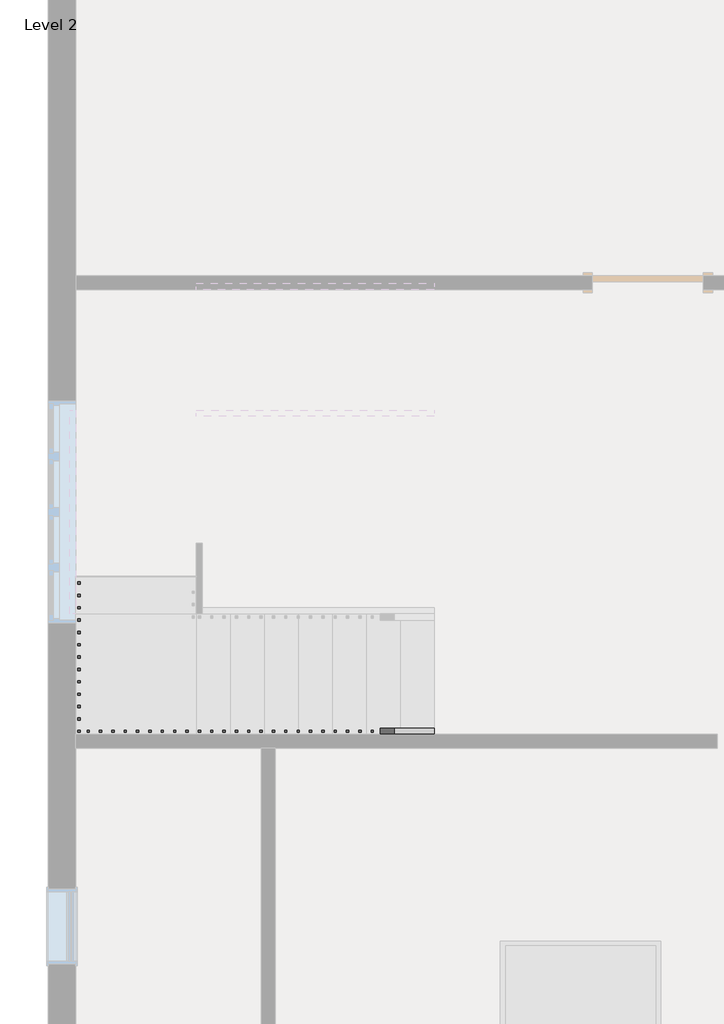
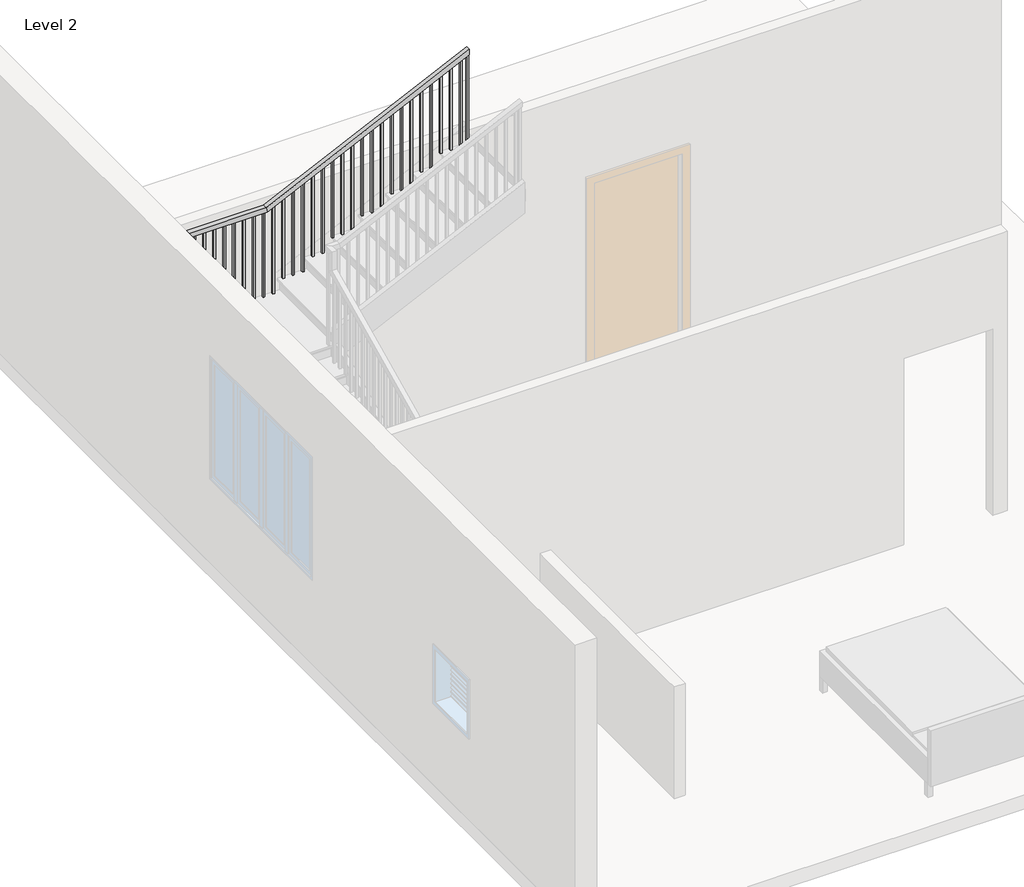
# One storey, part 2 of 3: 1 railing.
"""IFC4 building model written with IfcOpenShell, lengths in millimetres."""

from ifc_helpers import new_model, si_unit, frame, origin, place, context, project, spatial, polyline, outline, extrude, faceted_brep, element, save

model = new_model("IFC4")

# Units and contexts
model_context = context("Model", 3, world=origin())
ifc_project = project(units=[si_unit("LENGTHUNIT", "METRE", prefix="MILLI")], contexts=[model_context])

# Site, building, storey
site = spatial("IfcSite", under=ifc_project)
building = spatial("IfcBuilding", under=site)
storey = spatial("IfcBuildingStorey", under=building, Name="Level 2", Elevation=3048.0)

# Railing
placement = place(None, origin())
element("IfcRailing", 1, ObjectType="Handrail - Rectangular", at=placement, inside=storey, context=model_context, shape_type="SolidModel", body=[
    faceted_brep([(-19769.8789184, -1118.4399287, 4094.9217391), (-19769.8789184, -1118.4399287, 4038.6971684), (-19769.8789184, -1067.6399287, 4038.6971684), (-19769.8789184, -1067.6399287, 4094.9217391), (-21865.3789184, -1118.4399287, 5088.8347826), (-21876.8157218, -1118.4399287, 5038.0347826), (-21876.8157218, -1067.6399287, 5038.0347826), (-21865.3789184, -1067.6399287, 5088.8347826), (-22716.2789184, -1118.4399287, 5038.0347826), (-22716.2789184, -1118.4399287, 5088.8347826), (-22716.2789184, -267.5399287, 5088.8347826), (-22716.2789184, -256.1031254, 5038.0347826), (-22665.4789184, -1067.6399287, 5038.0347826), (-22665.4789184, -256.1031254, 5038.0347826), (-22665.4789184, -1067.6399287, 5088.8347826), (-22665.4789184, -267.5399287, 5088.8347826), (-22716.2789184, 2539.1600713, 5965.6869565), (-22716.2789184, 2539.1600713, 6016.4869565), (-21865.3789184, 2539.1600713, 6016.4869565), (-21853.9421151, 2539.1600713, 5965.6869565), (-22665.4789184, 2488.3600713, 5965.6869565), (-21853.9421151, 2488.3600713, 5965.6869565), (-22665.4789184, 2488.3600713, 6016.4869565), (-21865.3789184, 2488.3600713, 6016.4869565), (-22716.2789184, 1688.2600713, 6016.4869565), (-22716.2789184, 1699.6968746, 5965.6869565), (-22665.4789184, 1699.6968746, 5965.6869565), (-22665.4789184, 1688.2600713, 6016.4869565), (-19769.8789184, 2539.1600713, 7010.4), (-19769.8789184, 2488.3600713, 7010.4), (-19769.8789184, 2488.3600713, 6954.1754292), (-19769.8789184, 2539.1600713, 6954.1754292)], [[[0, 1, 2, 3]], [[1, 0, 4, 5]], [[2, 1, 5, 6]], [[3, 2, 6, 7]], [[0, 3, 7, 4]], [[8, 9, 10, 11]], [[12, 8, 11, 13]], [[14, 12, 13, 15]], [[9, 14, 15, 10]], [[16, 17, 18, 19]], [[20, 16, 19, 21]], [[22, 20, 21, 23]], [[17, 22, 23, 18]], [[5, 4, 9, 8]], [[6, 5, 8, 12]], [[7, 6, 12, 14]], [[4, 7, 14, 9]], [[11, 10, 24, 25]], [[13, 11, 25, 26]], [[15, 13, 26, 27]], [[10, 15, 27, 24]], [[25, 24, 17, 16]], [[26, 25, 16, 20]], [[27, 26, 20, 22]], [[24, 27, 22, 17]], [[28, 29, 30, 31]], [[19, 18, 28, 31]], [[21, 19, 31, 30]], [[23, 21, 30, 29]], [[18, 23, 29, 28]]]),
    extrude(outline(polyline([(6913.5153502, -19855.6039184), (5963.4782609, -19855.6039184), (5963.4782609, -19836.5539184), (6922.5509233, -19836.5539184), (6913.5153502, -19855.6039184)])), frame((0.0, 2504.2350713, 0.0), z_axis=(0.0, 1.0, 0.0), x_axis=(0.0, 0.0, 1.0)), (0.0, 0.0, 1.0), 19.05),
    extrude(outline(polyline([(6865.3256269, -19957.2039184), (5963.4782609, -19957.2039184), (5963.4782609, -19938.1539184), (6874.3612, -19938.1539184), (6865.3256269, -19957.2039184)])), frame((0.0, 2504.2350713, 0.0), z_axis=(0.0, 1.0, 0.0), x_axis=(0.0, 0.0, 1.0)), (0.0, 0.0, 1.0), 19.05),
    extrude(outline(polyline([(6817.1359035, -20058.8039184), (5963.4782609, -20058.8039184), (5963.4782609, -20039.7539184), (6826.1714767, -20039.7539184), (6817.1359035, -20058.8039184)])), frame((0.0, 2504.2350713, 0.0), z_axis=(0.0, 1.0, 0.0), x_axis=(0.0, 0.0, 1.0)), (0.0, 0.0, 1.0), 19.05),
    extrude(outline(polyline([(6768.9461802, -20160.4039184), (5830.9565217, -20160.4039184), (5830.9565217, -20141.3539184), (6777.9817533, -20141.3539184), (6768.9461802, -20160.4039184)])), frame((0.0, 2504.2350713, 0.0), z_axis=(0.0, 1.0, 0.0), x_axis=(0.0, 0.0, 1.0)), (0.0, 0.0, 1.0), 19.05),
    extrude(outline(polyline([(6720.7564569, -20262.0039184), (5830.9565217, -20262.0039184), (5830.9565217, -20242.9539184), (6729.79203, -20242.9539184), (6720.7564569, -20262.0039184)])), frame((0.0, 2504.2350713, 0.0), z_axis=(0.0, 1.0, 0.0), x_axis=(0.0, 0.0, 1.0)), (0.0, 0.0, 1.0), 19.05),
    extrude(outline(polyline([(6672.5667336, -20363.6039184), (5698.4347826, -20363.6039184), (5698.4347826, -20344.5539184), (6681.6023067, -20344.5539184), (6672.5667336, -20363.6039184)])), frame((0.0, 2504.2350713, 0.0), z_axis=(0.0, 1.0, 0.0), x_axis=(0.0, 0.0, 1.0)), (0.0, 0.0, 1.0), 19.05),
    extrude(outline(polyline([(6624.3770103, -20465.2039184), (5698.4347826, -20465.2039184), (5698.4347826, -20446.1539184), (6633.4125834, -20446.1539184), (6624.3770103, -20465.2039184)])), frame((0.0, 2504.2350713, 0.0), z_axis=(0.0, 1.0, 0.0), x_axis=(0.0, 0.0, 1.0)), (0.0, 0.0, 1.0), 19.05),
    extrude(outline(polyline([(6576.1872869, -20566.8039184), (5698.4347826, -20566.8039184), (5698.4347826, -20547.7539184), (6585.2228601, -20547.7539184), (6576.1872869, -20566.8039184)])), frame((0.0, 2504.2350713, 0.0), z_axis=(0.0, 1.0, 0.0), x_axis=(0.0, 0.0, 1.0)), (0.0, 0.0, 1.0), 19.05),
    extrude(outline(polyline([(6527.9975636, -20668.4039184), (5565.9130435, -20668.4039184), (5565.9130435, -20649.3539184), (6537.0331367, -20649.3539184), (6527.9975636, -20668.4039184)])), frame((0.0, 2504.2350713, 0.0), z_axis=(0.0, 1.0, 0.0), x_axis=(0.0, 0.0, 1.0)), (0.0, 0.0, 1.0), 19.05),
    extrude(outline(polyline([(6479.8078403, -20770.0039184), (5565.9130435, -20770.0039184), (5565.9130435, -20750.9539184), (6488.8434134, -20750.9539184), (6479.8078403, -20770.0039184)])), frame((0.0, 2504.2350713, 0.0), z_axis=(0.0, 1.0, 0.0), x_axis=(0.0, 0.0, 1.0)), (0.0, 0.0, 1.0), 19.05),
    extrude(outline(polyline([(6431.618117, -20871.6039184), (5565.9130435, -20871.6039184), (5565.9130435, -20852.5539184), (6440.6536901, -20852.5539184), (6431.618117, -20871.6039184)])), frame((0.0, 2504.2350713, 0.0), z_axis=(0.0, 1.0, 0.0), x_axis=(0.0, 0.0, 1.0)), (0.0, 0.0, 1.0), 19.05),
    extrude(outline(polyline([(6383.4283937, -20973.2039184), (5433.3913043, -20973.2039184), (5433.3913043, -20954.1539184), (6392.4639668, -20954.1539184), (6383.4283937, -20973.2039184)])), frame((0.0, 2504.2350713, 0.0), z_axis=(0.0, 1.0, 0.0), x_axis=(0.0, 0.0, 1.0)), (0.0, 0.0, 1.0), 19.05),
    extrude(outline(polyline([(6335.2386703, -21074.8039184), (5433.3913043, -21074.8039184), (5433.3913043, -21055.7539184), (6344.2742435, -21055.7539184), (6335.2386703, -21074.8039184)])), frame((0.0, 2504.2350713, 0.0), z_axis=(0.0, 1.0, 0.0), x_axis=(0.0, 0.0, 1.0)), (0.0, 0.0, 1.0), 19.05),
    extrude(outline(polyline([(6287.048947, -21176.4039184), (5433.3913043, -21176.4039184), (5433.3913043, -21157.3539184), (6296.0845201, -21157.3539184), (6287.048947, -21176.4039184)])), frame((0.0, 2504.2350713, 0.0), z_axis=(0.0, 1.0, 0.0), x_axis=(0.0, 0.0, 1.0)), (0.0, 0.0, 1.0), 19.05),
    extrude(outline(polyline([(6238.8592237, -21278.0039184), (5300.8695652, -21278.0039184), (5300.8695652, -21258.9539184), (6247.8947968, -21258.9539184), (6238.8592237, -21278.0039184)])), frame((0.0, 2504.2350713, 0.0), z_axis=(0.0, 1.0, 0.0), x_axis=(0.0, 0.0, 1.0)), (0.0, 0.0, 1.0), 19.05),
    extrude(outline(polyline([(6190.6695004, -21379.6039184), (5300.8695652, -21379.6039184), (5300.8695652, -21360.5539184), (6199.7050735, -21360.5539184), (6190.6695004, -21379.6039184)])), frame((0.0, 2504.2350713, 0.0), z_axis=(0.0, 1.0, 0.0), x_axis=(0.0, 0.0, 1.0)), (0.0, 0.0, 1.0), 19.05),
    extrude(outline(polyline([(6142.4797771, -21481.2039184), (5168.3478261, -21481.2039184), (5168.3478261, -21462.1539184), (6151.5153502, -21462.1539184), (6142.4797771, -21481.2039184)])), frame((0.0, 2504.2350713, 0.0), z_axis=(0.0, 1.0, 0.0), x_axis=(0.0, 0.0, 1.0)), (0.0, 0.0, 1.0), 19.05),
    extrude(outline(polyline([(6094.2900537, -21582.8039184), (5168.3478261, -21582.8039184), (5168.3478261, -21563.7539184), (6103.3256269, -21563.7539184), (6094.2900537, -21582.8039184)])), frame((0.0, 2504.2350713, 0.0), z_axis=(0.0, 1.0, 0.0), x_axis=(0.0, 0.0, 1.0)), (0.0, 0.0, 1.0), 19.05),
    extrude(outline(polyline([(6046.1003304, -21684.4039184), (5168.3478261, -21684.4039184), (5168.3478261, -21665.3539184), (6055.1359035, -21665.3539184), (6046.1003304, -21684.4039184)])), frame((0.0, 2504.2350713, 0.0), z_axis=(0.0, 1.0, 0.0), x_axis=(0.0, 0.0, 1.0)), (0.0, 0.0, 1.0), 19.05),
    extrude(outline(polyline([(5997.9106071, -21786.0039184), (5035.826087, -21786.0039184), (5035.826087, -21766.9539184), (6006.9461802, -21766.9539184), (5997.9106071, -21786.0039184)])), frame((0.0, 2504.2350713, 0.0), z_axis=(0.0, 1.0, 0.0), x_axis=(0.0, 0.0, 1.0)), (0.0, 0.0, 1.0), 19.05),
    extrude(outline(polyline([(-21887.6039184, 2523.2850713), (-21868.5539184, 2523.2850713), (-21868.5539184, 2504.2350713), (-21887.6039184, 2504.2350713), (-21887.6039184, 2523.2850713)])), frame((0.0, 0.0, 5035.826087), z_axis=(0.0, 0.0, 1.0), x_axis=(1.0, 0.0, 0.0)), (0.0, 0.0, 1.0), 929.8608696),
    extrude(outline(polyline([(-21989.2039184, 2523.2850713), (-21970.1539184, 2523.2850713), (-21970.1539184, 2504.2350713), (-21989.2039184, 2504.2350713), (-21989.2039184, 2523.2850713)])), frame((0.0, 0.0, 5035.826087), z_axis=(0.0, 0.0, 1.0), x_axis=(1.0, 0.0, 0.0)), (0.0, 0.0, 1.0), 929.8608696),
    extrude(outline(polyline([(-22090.8039184, 2523.2850713), (-22071.7539184, 2523.2850713), (-22071.7539184, 2504.2350713), (-22090.8039184, 2504.2350713), (-22090.8039184, 2523.2850713)])), frame((0.0, 0.0, 5035.826087), z_axis=(0.0, 0.0, 1.0), x_axis=(1.0, 0.0, 0.0)), (0.0, 0.0, 1.0), 929.8608696),
    extrude(outline(polyline([(-22192.4039184, 2523.2850713), (-22173.3539184, 2523.2850713), (-22173.3539184, 2504.2350713), (-22192.4039184, 2504.2350713), (-22192.4039184, 2523.2850713)])), frame((0.0, 0.0, 5035.826087), z_axis=(0.0, 0.0, 1.0), x_axis=(1.0, 0.0, 0.0)), (0.0, 0.0, 1.0), 929.8608696),
    extrude(outline(polyline([(-22294.0039184, 2523.2850713), (-22274.9539184, 2523.2850713), (-22274.9539184, 2504.2350713), (-22294.0039184, 2504.2350713), (-22294.0039184, 2523.2850713)])), frame((0.0, 0.0, 5035.826087), z_axis=(0.0, 0.0, 1.0), x_axis=(1.0, 0.0, 0.0)), (0.0, 0.0, 1.0), 929.8608696),
    extrude(outline(polyline([(-22395.6039184, 2523.2850713), (-22376.5539184, 2523.2850713), (-22376.5539184, 2504.2350713), (-22395.6039184, 2504.2350713), (-22395.6039184, 2523.2850713)])), frame((0.0, 0.0, 5035.826087), z_axis=(0.0, 0.0, 1.0), x_axis=(1.0, 0.0, 0.0)), (0.0, 0.0, 1.0), 929.8608696),
    extrude(outline(polyline([(-22497.2039184, 2523.2850713), (-22478.1539184, 2523.2850713), (-22478.1539184, 2504.2350713), (-22497.2039184, 2504.2350713), (-22497.2039184, 2523.2850713)])), frame((0.0, 0.0, 5035.826087), z_axis=(0.0, 0.0, 1.0), x_axis=(1.0, 0.0, 0.0)), (0.0, 0.0, 1.0), 929.8608696),
    extrude(outline(polyline([(-22598.8039184, 2523.2850713), (-22579.7539184, 2523.2850713), (-22579.7539184, 2504.2350713), (-22598.8039184, 2504.2350713), (-22598.8039184, 2523.2850713)])), frame((0.0, 0.0, 5035.826087), z_axis=(0.0, 0.0, 1.0), x_axis=(1.0, 0.0, 0.0)), (0.0, 0.0, 1.0), 929.8608696),
    extrude(outline(polyline([(-22700.4039184, 2453.4350713), (-22700.4039184, 2472.4850713), (-22681.3539184, 2472.4850713), (-22681.3539184, 2453.4350713), (-22700.4039184, 2453.4350713)])), frame((0.0, 0.0, 5035.826087), z_axis=(0.0, 0.0, 1.0), x_axis=(1.0, 0.0, 0.0)), (0.0, 0.0, 1.0), 929.8608696),
    extrude(outline(polyline([(-22700.4039184, 2351.8350713), (-22700.4039184, 2370.8850713), (-22681.3539184, 2370.8850713), (-22681.3539184, 2351.8350713), (-22700.4039184, 2351.8350713)])), frame((0.0, 0.0, 5035.826087), z_axis=(0.0, 0.0, 1.0), x_axis=(1.0, 0.0, 0.0)), (0.0, 0.0, 1.0), 929.8608696),
    extrude(outline(polyline([(-22700.4039184, 2250.2350713), (-22700.4039184, 2269.2850713), (-22681.3539184, 2269.2850713), (-22681.3539184, 2250.2350713), (-22700.4039184, 2250.2350713)])), frame((0.0, 0.0, 5035.826087), z_axis=(0.0, 0.0, 1.0), x_axis=(1.0, 0.0, 0.0)), (0.0, 0.0, 1.0), 929.8608696),
    extrude(outline(polyline([(-22700.4039184, 2148.6350713), (-22700.4039184, 2167.6850713), (-22681.3539184, 2167.6850713), (-22681.3539184, 2148.6350713), (-22700.4039184, 2148.6350713)])), frame((0.0, 0.0, 5035.826087), z_axis=(0.0, 0.0, 1.0), x_axis=(1.0, 0.0, 0.0)), (0.0, 0.0, 1.0), 929.8608696),
    extrude(outline(polyline([(-22700.4039184, 2047.0350713), (-22700.4039184, 2066.0850713), (-22681.3539184, 2066.0850713), (-22681.3539184, 2047.0350713), (-22700.4039184, 2047.0350713)])), frame((0.0, 0.0, 5035.826087), z_axis=(0.0, 0.0, 1.0), x_axis=(1.0, 0.0, 0.0)), (0.0, 0.0, 1.0), 929.8608696),
    extrude(outline(polyline([(-22700.4039184, 1945.4350713), (-22700.4039184, 1964.4850713), (-22681.3539184, 1964.4850713), (-22681.3539184, 1945.4350713), (-22700.4039184, 1945.4350713)])), frame((0.0, 0.0, 5035.826087), z_axis=(0.0, 0.0, 1.0), x_axis=(1.0, 0.0, 0.0)), (0.0, 0.0, 1.0), 929.8608696),
    extrude(outline(polyline([(-22700.4039184, 1843.8350713), (-22700.4039184, 1862.8850713), (-22681.3539184, 1862.8850713), (-22681.3539184, 1843.8350713), (-22700.4039184, 1843.8350713)])), frame((0.0, 0.0, 5035.826087), z_axis=(0.0, 0.0, 1.0), x_axis=(1.0, 0.0, 0.0)), (0.0, 0.0, 1.0), 929.8608696),
    extrude(outline(polyline([(-22700.4039184, 1742.2350713), (-22700.4039184, 1761.2850713), (-22681.3539184, 1761.2850713), (-22681.3539184, 1742.2350713), (-22700.4039184, 1742.2350713)])), frame((0.0, 0.0, 5035.826087), z_axis=(0.0, 0.0, 1.0), x_axis=(1.0, 0.0, 0.0)), (0.0, 0.0, 1.0), 929.8608696),
    extrude(outline(polyline([(1659.6850713, 5946.7090261), (1659.6850713, 5035.826087), (1640.6350713, 5035.826087), (1640.6350713, 5937.6734529), (1659.6850713, 5946.7090261)])), frame((-22700.4039184, 0.0, 0.0), z_axis=(1.0, 0.0, 0.0), x_axis=(0.0, 1.0, 0.0)), (0.0, 0.0, 1.0), 19.05),
    extrude(outline(polyline([(1558.0850713, 5898.5193027), (1558.0850713, 5035.826087), (1539.0350713, 5035.826087), (1539.0350713, 5889.4837296), (1558.0850713, 5898.5193027)])), frame((-22700.4039184, 0.0, 0.0), z_axis=(1.0, 0.0, 0.0), x_axis=(0.0, 1.0, 0.0)), (0.0, 0.0, 1.0), 19.05),
    extrude(outline(polyline([(1456.4850713, 5850.3295794), (1456.4850713, 4903.3043478), (1437.4350713, 4903.3043478), (1437.4350713, 5841.2940063), (1456.4850713, 5850.3295794)])), frame((-22700.4039184, 0.0, 0.0), z_axis=(1.0, 0.0, 0.0), x_axis=(0.0, 1.0, 0.0)), (0.0, 0.0, 1.0), 19.05),
    extrude(outline(polyline([(1354.8850713, 5802.1398561), (1354.8850713, 4903.3043478), (1335.8350713, 4903.3043478), (1335.8350713, 5793.104283), (1354.8850713, 5802.1398561)])), frame((-22700.4039184, 0.0, 0.0), z_axis=(1.0, 0.0, 0.0), x_axis=(0.0, 1.0, 0.0)), (0.0, 0.0, 1.0), 19.05),
    extrude(outline(polyline([(1253.2850713, 5753.9501328), (1253.2850713, 4770.7826087), (1234.2350713, 4770.7826087), (1234.2350713, 5744.9145597), (1253.2850713, 5753.9501328)])), frame((-22700.4039184, 0.0, 0.0), z_axis=(1.0, 0.0, 0.0), x_axis=(0.0, 1.0, 0.0)), (0.0, 0.0, 1.0), 19.05),
    extrude(outline(polyline([(1151.6850713, 5705.7604095), (1151.6850713, 4770.7826087), (1132.6350713, 4770.7826087), (1132.6350713, 5696.7248363), (1151.6850713, 5705.7604095)])), frame((-22700.4039184, 0.0, 0.0), z_axis=(1.0, 0.0, 0.0), x_axis=(0.0, 1.0, 0.0)), (0.0, 0.0, 1.0), 19.05),
    extrude(outline(polyline([(1050.0850713, 5657.5706861), (1050.0850713, 4770.7826087), (1031.0350713, 4770.7826087), (1031.0350713, 5648.535113), (1050.0850713, 5657.5706861)])), frame((-22700.4039184, 0.0, 0.0), z_axis=(1.0, 0.0, 0.0), x_axis=(0.0, 1.0, 0.0)), (0.0, 0.0, 1.0), 19.05),
    extrude(outline(polyline([(948.4850713, 5609.3809628), (948.4850713, 4638.2608696), (929.4350713, 4638.2608696), (929.4350713, 5600.3453897), (948.4850713, 5609.3809628)])), frame((-22700.4039184, 0.0, 0.0), z_axis=(1.0, 0.0, 0.0), x_axis=(0.0, 1.0, 0.0)), (0.0, 0.0, 1.0), 19.05),
    extrude(outline(polyline([(846.8850713, 5561.1912395), (846.8850713, 4638.2608696), (827.8350713, 4638.2608696), (827.8350713, 5552.1556664), (846.8850713, 5561.1912395)])), frame((-22700.4039184, 0.0, 0.0), z_axis=(1.0, 0.0, 0.0), x_axis=(0.0, 1.0, 0.0)), (0.0, 0.0, 1.0), 19.05),
    extrude(outline(polyline([(745.2850713, 5513.0015162), (745.2850713, 4638.2608696), (726.2350713, 4638.2608696), (726.2350713, 5503.9659431), (745.2850713, 5513.0015162)])), frame((-22700.4039184, 0.0, 0.0), z_axis=(1.0, 0.0, 0.0), x_axis=(0.0, 1.0, 0.0)), (0.0, 0.0, 1.0), 19.05),
    extrude(outline(polyline([(643.6850713, 5464.8117929), (643.6850713, 4505.7391304), (624.6350713, 4505.7391304), (624.6350713, 5455.7762197), (643.6850713, 5464.8117929)])), frame((-22700.4039184, 0.0, 0.0), z_axis=(1.0, 0.0, 0.0), x_axis=(0.0, 1.0, 0.0)), (0.0, 0.0, 1.0), 19.05),
    extrude(outline(polyline([(542.0850713, 5416.6220695), (542.0850713, 4505.7391304), (523.0350713, 4505.7391304), (523.0350713, 5407.5864964), (542.0850713, 5416.6220695)])), frame((-22700.4039184, 0.0, 0.0), z_axis=(1.0, 0.0, 0.0), x_axis=(0.0, 1.0, 0.0)), (0.0, 0.0, 1.0), 19.05),
    extrude(outline(polyline([(440.4850713, 5368.4323462), (440.4850713, 4505.7391304), (421.4350713, 4505.7391304), (421.4350713, 5359.3967731), (440.4850713, 5368.4323462)])), frame((-22700.4039184, 0.0, 0.0), z_axis=(1.0, 0.0, 0.0), x_axis=(0.0, 1.0, 0.0)), (0.0, 0.0, 1.0), 19.05),
    extrude(outline(polyline([(338.8850713, 5320.2426229), (338.8850713, 4373.2173913), (319.8350713, 4373.2173913), (319.8350713, 5311.2070498), (338.8850713, 5320.2426229)])), frame((-22700.4039184, 0.0, 0.0), z_axis=(1.0, 0.0, 0.0), x_axis=(0.0, 1.0, 0.0)), (0.0, 0.0, 1.0), 19.05),
    extrude(outline(polyline([(237.2850713, 5272.0528996), (237.2850713, 4373.2173913), (218.2350713, 4373.2173913), (218.2350713, 5263.0173265), (237.2850713, 5272.0528996)])), frame((-22700.4039184, 0.0, 0.0), z_axis=(1.0, 0.0, 0.0), x_axis=(0.0, 1.0, 0.0)), (0.0, 0.0, 1.0), 19.05),
    extrude(outline(polyline([(135.6850713, 5223.8631763), (135.6850713, 4240.6956522), (116.6350713, 4240.6956522), (116.6350713, 5214.8276031), (135.6850713, 5223.8631763)])), frame((-22700.4039184, 0.0, 0.0), z_axis=(1.0, 0.0, 0.0), x_axis=(0.0, 1.0, 0.0)), (0.0, 0.0, 1.0), 19.05),
    extrude(outline(polyline([(34.0850713, 5175.6734529), (34.0850713, 4240.6956522), (15.0350713, 4240.6956522), (15.0350713, 5166.6378798), (34.0850713, 5175.6734529)])), frame((-22700.4039184, 0.0, 0.0), z_axis=(1.0, 0.0, 0.0), x_axis=(0.0, 1.0, 0.0)), (0.0, 0.0, 1.0), 19.05),
    extrude(outline(polyline([(-67.5149287, 5127.4837296), (-67.5149287, 4240.6956522), (-86.5649287, 4240.6956522), (-86.5649287, 5118.4481565), (-67.5149287, 5127.4837296)])), frame((-22700.4039184, 0.0, 0.0), z_axis=(1.0, 0.0, 0.0), x_axis=(0.0, 1.0, 0.0)), (0.0, 0.0, 1.0), 19.05),
    extrude(outline(polyline([(-169.1149287, 5079.2940063), (-169.1149287, 4108.173913), (-188.1649287, 4108.173913), (-188.1649287, 5070.2584332), (-169.1149287, 5079.2940063)])), frame((-22700.4039184, 0.0, 0.0), z_axis=(1.0, 0.0, 0.0), x_axis=(0.0, 1.0, 0.0)), (0.0, 0.0, 1.0), 19.05),
    extrude(outline(polyline([(-22700.4039184, -289.7649287), (-22700.4039184, -270.7149287), (-22681.3539184, -270.7149287), (-22681.3539184, -289.7649287), (-22700.4039184, -289.7649287)])), frame((0.0, 0.0, 4108.173913), z_axis=(0.0, 0.0, 1.0), x_axis=(1.0, 0.0, 0.0)), (0.0, 0.0, 1.0), 929.8608696),
    extrude(outline(polyline([(-22700.4039184, -391.3649287), (-22700.4039184, -372.3149287), (-22681.3539184, -372.3149287), (-22681.3539184, -391.3649287), (-22700.4039184, -391.3649287)])), frame((0.0, 0.0, 4108.173913), z_axis=(0.0, 0.0, 1.0), x_axis=(1.0, 0.0, 0.0)), (0.0, 0.0, 1.0), 929.8608696),
    extrude(outline(polyline([(-22700.4039184, -492.9649287), (-22700.4039184, -473.9149287), (-22681.3539184, -473.9149287), (-22681.3539184, -492.9649287), (-22700.4039184, -492.9649287)])), frame((0.0, 0.0, 4108.173913), z_axis=(0.0, 0.0, 1.0), x_axis=(1.0, 0.0, 0.0)), (0.0, 0.0, 1.0), 929.8608696),
    extrude(outline(polyline([(-22700.4039184, -594.5649287), (-22700.4039184, -575.5149287), (-22681.3539184, -575.5149287), (-22681.3539184, -594.5649287), (-22700.4039184, -594.5649287)])), frame((0.0, 0.0, 4108.173913), z_axis=(0.0, 0.0, 1.0), x_axis=(1.0, 0.0, 0.0)), (0.0, 0.0, 1.0), 929.8608696),
    extrude(outline(polyline([(-22700.4039184, -696.1649287), (-22700.4039184, -677.1149287), (-22681.3539184, -677.1149287), (-22681.3539184, -696.1649287), (-22700.4039184, -696.1649287)])), frame((0.0, 0.0, 4108.173913), z_axis=(0.0, 0.0, 1.0), x_axis=(1.0, 0.0, 0.0)), (0.0, 0.0, 1.0), 929.8608696),
    extrude(outline(polyline([(-22700.4039184, -797.7649287), (-22700.4039184, -778.7149287), (-22681.3539184, -778.7149287), (-22681.3539184, -797.7649287), (-22700.4039184, -797.7649287)])), frame((0.0, 0.0, 4108.173913), z_axis=(0.0, 0.0, 1.0), x_axis=(1.0, 0.0, 0.0)), (0.0, 0.0, 1.0), 929.8608696),
    extrude(outline(polyline([(-22700.4039184, -899.3649287), (-22700.4039184, -880.3149287), (-22681.3539184, -880.3149287), (-22681.3539184, -899.3649287), (-22700.4039184, -899.3649287)])), frame((0.0, 0.0, 4108.173913), z_axis=(0.0, 0.0, 1.0), x_axis=(1.0, 0.0, 0.0)), (0.0, 0.0, 1.0), 929.8608696),
    extrude(outline(polyline([(-22700.4039184, -1000.9649287), (-22700.4039184, -981.9149287), (-22681.3539184, -981.9149287), (-22681.3539184, -1000.9649287), (-22700.4039184, -1000.9649287)])), frame((0.0, 0.0, 4108.173913), z_axis=(0.0, 0.0, 1.0), x_axis=(1.0, 0.0, 0.0)), (0.0, 0.0, 1.0), 929.8608696),
    extrude(outline(polyline([(-22605.1539184, -1102.5649287), (-22624.2039184, -1102.5649287), (-22624.2039184, -1083.5149287), (-22605.1539184, -1083.5149287), (-22605.1539184, -1102.5649287)])), frame((0.0, 0.0, 4108.173913), z_axis=(0.0, 0.0, 1.0), x_axis=(1.0, 0.0, 0.0)), (0.0, 0.0, 1.0), 929.8608696),
    extrude(outline(polyline([(-22503.5539184, -1102.5649287), (-22522.6039184, -1102.5649287), (-22522.6039184, -1083.5149287), (-22503.5539184, -1083.5149287), (-22503.5539184, -1102.5649287)])), frame((0.0, 0.0, 4108.173913), z_axis=(0.0, 0.0, 1.0), x_axis=(1.0, 0.0, 0.0)), (0.0, 0.0, 1.0), 929.8608696),
    extrude(outline(polyline([(-22401.9539184, -1102.5649287), (-22421.0039184, -1102.5649287), (-22421.0039184, -1083.5149287), (-22401.9539184, -1083.5149287), (-22401.9539184, -1102.5649287)])), frame((0.0, 0.0, 4108.173913), z_axis=(0.0, 0.0, 1.0), x_axis=(1.0, 0.0, 0.0)), (0.0, 0.0, 1.0), 929.8608696),
    extrude(outline(polyline([(-22300.3539184, -1102.5649287), (-22319.4039184, -1102.5649287), (-22319.4039184, -1083.5149287), (-22300.3539184, -1083.5149287), (-22300.3539184, -1102.5649287)])), frame((0.0, 0.0, 4108.173913), z_axis=(0.0, 0.0, 1.0), x_axis=(1.0, 0.0, 0.0)), (0.0, 0.0, 1.0), 929.8608696),
    extrude(outline(polyline([(-22198.7539184, -1102.5649287), (-22217.8039184, -1102.5649287), (-22217.8039184, -1083.5149287), (-22198.7539184, -1083.5149287), (-22198.7539184, -1102.5649287)])), frame((0.0, 0.0, 4108.173913), z_axis=(0.0, 0.0, 1.0), x_axis=(1.0, 0.0, 0.0)), (0.0, 0.0, 1.0), 929.8608696),
    extrude(outline(polyline([(-22097.1539184, -1102.5649287), (-22116.2039184, -1102.5649287), (-22116.2039184, -1083.5149287), (-22097.1539184, -1083.5149287), (-22097.1539184, -1102.5649287)])), frame((0.0, 0.0, 4108.173913), z_axis=(0.0, 0.0, 1.0), x_axis=(1.0, 0.0, 0.0)), (0.0, 0.0, 1.0), 929.8608696),
    extrude(outline(polyline([(-21995.5539184, -1102.5649287), (-22014.6039184, -1102.5649287), (-22014.6039184, -1083.5149287), (-21995.5539184, -1083.5149287), (-21995.5539184, -1102.5649287)])), frame((0.0, 0.0, 4108.173913), z_axis=(0.0, 0.0, 1.0), x_axis=(1.0, 0.0, 0.0)), (0.0, 0.0, 1.0), 929.8608696),
    extrude(outline(polyline([(-21893.9539184, -1102.5649287), (-21913.0039184, -1102.5649287), (-21913.0039184, -1083.5149287), (-21893.9539184, -1083.5149287), (-21893.9539184, -1102.5649287)])), frame((0.0, 0.0, 4108.173913), z_axis=(0.0, 0.0, 1.0), x_axis=(1.0, 0.0, 0.0)), (0.0, 0.0, 1.0), 929.8608696),
    extrude(outline(polyline([(5007.0094213, -21811.4039184), (4108.173913, -21811.4039184), (4108.173913, -21792.3539184), (4997.9738482, -21792.3539184), (5007.0094213, -21811.4039184)])), frame((0.0, -1102.5649287, 0.0), z_axis=(0.0, 1.0, 0.0), x_axis=(0.0, 0.0, 1.0)), (0.0, 0.0, 1.0), 19.05),
    extrude(outline(polyline([(4958.819698, -21709.8039184), (3975.6521739, -21709.8039184), (3975.6521739, -21690.7539184), (4949.7841249, -21690.7539184), (4958.819698, -21709.8039184)])), frame((0.0, -1102.5649287, 0.0), z_axis=(0.0, 1.0, 0.0), x_axis=(0.0, 0.0, 1.0)), (0.0, 0.0, 1.0), 19.05),
    extrude(outline(polyline([(4910.6299747, -21608.2039184), (3975.6521739, -21608.2039184), (3975.6521739, -21589.1539184), (4901.5944016, -21589.1539184), (4910.6299747, -21608.2039184)])), frame((0.0, -1102.5649287, 0.0), z_axis=(0.0, 1.0, 0.0), x_axis=(0.0, 0.0, 1.0)), (0.0, 0.0, 1.0), 19.05),
    extrude(outline(polyline([(4862.4402514, -21506.6039184), (3975.6521739, -21506.6039184), (3975.6521739, -21487.5539184), (4853.4046782, -21487.5539184), (4862.4402514, -21506.6039184)])), frame((0.0, -1102.5649287, 0.0), z_axis=(0.0, 1.0, 0.0), x_axis=(0.0, 0.0, 1.0)), (0.0, 0.0, 1.0), 19.05),
    extrude(outline(polyline([(4814.250528, -21405.0039184), (3843.1304348, -21405.0039184), (3843.1304348, -21385.9539184), (4805.2149549, -21385.9539184), (4814.250528, -21405.0039184)])), frame((0.0, -1102.5649287, 0.0), z_axis=(0.0, 1.0, 0.0), x_axis=(0.0, 0.0, 1.0)), (0.0, 0.0, 1.0), 19.05),
    extrude(outline(polyline([(4766.0608047, -21303.4039184), (3843.1304348, -21303.4039184), (3843.1304348, -21284.3539184), (4757.0252316, -21284.3539184), (4766.0608047, -21303.4039184)])), frame((0.0, -1102.5649287, 0.0), z_axis=(0.0, 1.0, 0.0), x_axis=(0.0, 0.0, 1.0)), (0.0, 0.0, 1.0), 19.05),
    extrude(outline(polyline([(4717.8710814, -21201.8039184), (3843.1304348, -21201.8039184), (3843.1304348, -21182.7539184), (4708.8355083, -21182.7539184), (4717.8710814, -21201.8039184)])), frame((0.0, -1102.5649287, 0.0), z_axis=(0.0, 1.0, 0.0), x_axis=(0.0, 0.0, 1.0)), (0.0, 0.0, 1.0), 19.05),
    extrude(outline(polyline([(4669.6813581, -21100.2039184), (3710.6086957, -21100.2039184), (3710.6086957, -21081.1539184), (4660.645785, -21081.1539184), (4669.6813581, -21100.2039184)])), frame((0.0, -1102.5649287, 0.0), z_axis=(0.0, 1.0, 0.0), x_axis=(0.0, 0.0, 1.0)), (0.0, 0.0, 1.0), 19.05),
    extrude(outline(polyline([(4621.4916348, -20998.6039184), (3710.6086957, -20998.6039184), (3710.6086957, -20979.5539184), (4612.4560616, -20979.5539184), (4621.4916348, -20998.6039184)])), frame((0.0, -1102.5649287, 0.0), z_axis=(0.0, 1.0, 0.0), x_axis=(0.0, 0.0, 1.0)), (0.0, 0.0, 1.0), 19.05),
    extrude(outline(polyline([(4573.3019114, -20897.0039184), (3710.6086957, -20897.0039184), (3710.6086957, -20877.9539184), (4564.2663383, -20877.9539184), (4573.3019114, -20897.0039184)])), frame((0.0, -1102.5649287, 0.0), z_axis=(0.0, 1.0, 0.0), x_axis=(0.0, 0.0, 1.0)), (0.0, 0.0, 1.0), 19.05),
    extrude(outline(polyline([(4525.1121881, -20795.4039184), (3578.0869565, -20795.4039184), (3578.0869565, -20776.3539184), (4516.076615, -20776.3539184), (4525.1121881, -20795.4039184)])), frame((0.0, -1102.5649287, 0.0), z_axis=(0.0, 1.0, 0.0), x_axis=(0.0, 0.0, 1.0)), (0.0, 0.0, 1.0), 19.05),
    extrude(outline(polyline([(4476.9224648, -20693.8039184), (3578.0869565, -20693.8039184), (3578.0869565, -20674.7539184), (4467.8868917, -20674.7539184), (4476.9224648, -20693.8039184)])), frame((0.0, -1102.5649287, 0.0), z_axis=(0.0, 1.0, 0.0), x_axis=(0.0, 0.0, 1.0)), (0.0, 0.0, 1.0), 19.05),
    extrude(outline(polyline([(4428.7327415, -20592.2039184), (3445.5652174, -20592.2039184), (3445.5652174, -20573.1539184), (4419.6971684, -20573.1539184), (4428.7327415, -20592.2039184)])), frame((0.0, -1102.5649287, 0.0), z_axis=(0.0, 1.0, 0.0), x_axis=(0.0, 0.0, 1.0)), (0.0, 0.0, 1.0), 19.05),
    extrude(outline(polyline([(4380.5430182, -20490.6039184), (3445.5652174, -20490.6039184), (3445.5652174, -20471.5539184), (4371.507445, -20471.5539184), (4380.5430182, -20490.6039184)])), frame((0.0, -1102.5649287, 0.0), z_axis=(0.0, 1.0, 0.0), x_axis=(0.0, 0.0, 1.0)), (0.0, 0.0, 1.0), 19.05),
    extrude(outline(polyline([(4332.3532948, -20389.0039184), (3445.5652174, -20389.0039184), (3445.5652174, -20369.9539184), (4323.3177217, -20369.9539184), (4332.3532948, -20389.0039184)])), frame((0.0, -1102.5649287, 0.0), z_axis=(0.0, 1.0, 0.0), x_axis=(0.0, 0.0, 1.0)), (0.0, 0.0, 1.0), 19.05),
    extrude(outline(polyline([(4284.1635715, -20287.4039184), (3313.0434783, -20287.4039184), (3313.0434783, -20268.3539184), (4275.1279984, -20268.3539184), (4284.1635715, -20287.4039184)])), frame((0.0, -1102.5649287, 0.0), z_axis=(0.0, 1.0, 0.0), x_axis=(0.0, 0.0, 1.0)), (0.0, 0.0, 1.0), 19.05),
    extrude(outline(polyline([(4235.9738482, -20185.8039184), (3313.0434783, -20185.8039184), (3313.0434783, -20166.7539184), (4226.9382751, -20166.7539184), (4235.9738482, -20185.8039184)])), frame((0.0, -1102.5649287, 0.0), z_axis=(0.0, 1.0, 0.0), x_axis=(0.0, 0.0, 1.0)), (0.0, 0.0, 1.0), 19.05),
    extrude(outline(polyline([(4187.7841249, -20084.2039184), (3313.0434783, -20084.2039184), (3313.0434783, -20065.1539184), (4178.7485518, -20065.1539184), (4187.7841249, -20084.2039184)])), frame((0.0, -1102.5649287, 0.0), z_axis=(0.0, 1.0, 0.0), x_axis=(0.0, 0.0, 1.0)), (0.0, 0.0, 1.0), 19.05),
    extrude(outline(polyline([(4139.5944016, -19982.6039184), (3180.5217391, -19982.6039184), (3180.5217391, -19963.5539184), (4130.5588284, -19963.5539184), (4139.5944016, -19982.6039184)])), frame((0.0, -1102.5649287, 0.0), z_axis=(0.0, 1.0, 0.0), x_axis=(0.0, 0.0, 1.0)), (0.0, 0.0, 1.0), 19.05),
    extrude(outline(polyline([(4091.4046782, -19881.0039184), (3180.5217391, -19881.0039184), (3180.5217391, -19861.9539184), (4082.3691051, -19861.9539184), (4091.4046782, -19881.0039184)])), frame((0.0, -1102.5649287, 0.0), z_axis=(0.0, 1.0, 0.0), x_axis=(0.0, 0.0, 1.0)), (0.0, 0.0, 1.0), 19.05),
    extrude(outline(polyline([(-22700.4039184, 2504.2350713), (-22700.4039184, 2523.2850713), (-22681.3539184, 2523.2850713), (-22681.3539184, 2504.2350713), (-22700.4039184, 2504.2350713)])), frame((0.0, 0.0, 5035.826087), z_axis=(0.0, 0.0, 1.0), x_axis=(1.0, 0.0, 0.0)), (0.0, 0.0, 1.0), 929.8608696),
    extrude(outline(polyline([(-22681.3539184, -1102.5649287), (-22700.4039184, -1102.5649287), (-22700.4039184, -1083.5149287), (-22681.3539184, -1083.5149287), (-22681.3539184, -1102.5649287)])), frame((0.0, 0.0, 4108.173913), z_axis=(0.0, 0.0, 1.0), x_axis=(1.0, 0.0, 0.0)), (0.0, 0.0, 1.0), 929.8608696),
    extrude(outline(polyline([(6945.1398561, -19788.9289184), (5963.4782609, -19788.9289184), (5963.4782609, -19769.8789184), (6954.1754292, -19769.8789184), (6945.1398561, -19788.9289184)])), frame((0.0, 2504.2350713, 0.0), z_axis=(0.0, 1.0, 0.0), x_axis=(0.0, 0.0, 1.0)), (0.0, 0.0, 1.0), 19.05),
    extrude(outline(polyline([(4047.7327415, -19788.9289184), (3180.5217391, -19788.9289184), (3180.5217391, -19769.8789184), (4038.6971684, -19769.8789184), (4047.7327415, -19788.9289184)])), frame((0.0, -1102.5649287, 0.0), z_axis=(0.0, 1.0, 0.0), x_axis=(0.0, 0.0, 1.0)), (0.0, 0.0, 1.0), 19.05),
])

save(model, "model.ifc")

# Revit data of these elements
# Type "Handrail - Rectangular"
#   Assembly Code = "C2010400"
#   built-in parameter 1008612 = 0.0416667 (stored number, unit not read)
#   built-in parameter 1008611 = 0.0416667 (stored number, unit not read)
#   built-in parameter 1008609 = 0.333333 (stored number, unit not read)
#   built-in parameter 1008604 = 0.166667 (stored number, unit not read)
#   built-in parameter 1008603 = 0.166667 (stored number, unit not read)
#   Railing Height = 3' - 0"
#   built-in parameter 1008630 = 2
#   built-in parameter 1008610 = 2
#   built-in parameter 1008618 = Baluster - Square : 3/4"
# Element 1 (IfcRailing, "Handrail - Rectangular")
#   Phase Created = New Construction
